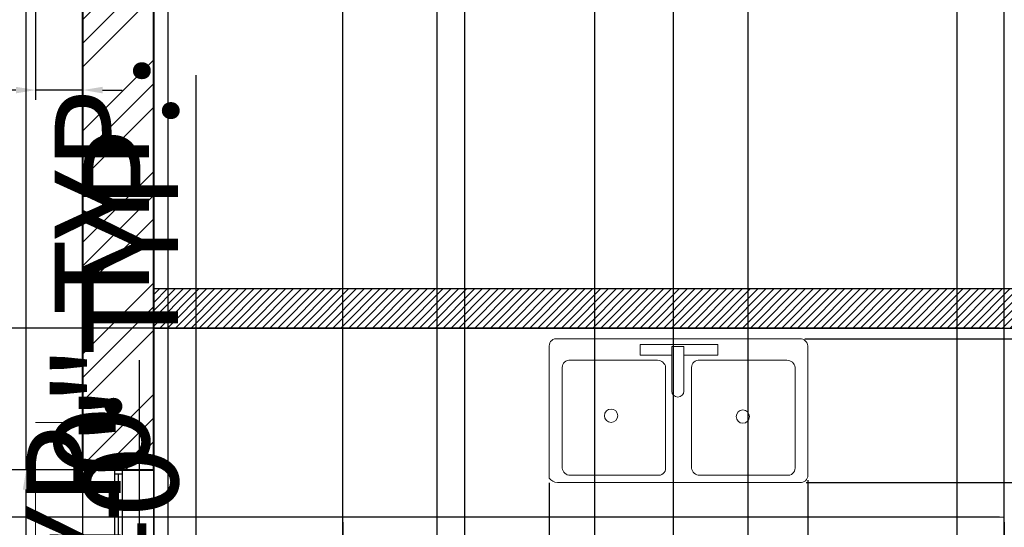
# Model space of a CAD drawing. Units: inches. Extents: x 2386 to 3029, y 792 to 1465.
# Tile 8 of 12: x 2463 to 2588, y 1205 to 1269. Entities that reach past the tile are written whole.
import ezdxf

# ---------------------------------------------------------------- set-up
doc = ezdxf.new("R2010")
doc.units = ezdxf.units.IN
doc.linetypes.add('ACAD_ISO02W100', pattern=[15, 12, -3])
for name, color, linetype, lineweight in [('A-DIMS', 1, 'Continuous', 18), ('A-FLOR-CASE', 6, 'Continuous', 18), ('A-FLOR-FIXT', 9, 'Continuous', 18), ('A-WALL-EXT', 7, 'Continuous', 40), ('A-WALL-INT', 9, 'Continuous', 30), ('A-WALL-PATT', 9, 'Continuous', 13), ('A-WINDOW', 4, 'Continuous', 25), ('A-WINDOW-OVHD', 4, 'ACAD_ISO02W100', 18)]:
    doc.layers.add(name, color=color, linetype=linetype, lineweight=lineweight)
doc.styles.get("Standard").update_dxf_attribs({"font": 'arial.ttf'})
doc.dimstyles.new('ISO-25', dxfattribs={"dimtxt": 12, "dimasz": 2.5, "dimexe": 1.25, "dimexo": 0.625, "dimtad": 1, "dimlunit": 4, "dimtxsty": 'Standard', "dimcen": 2.5, "dimadec": 0, "dimazin": 0, "dimtfac": 1, "dimtmove": 0, "dimatfit": 3, "dimfxl": 1, "dimarcsym": 0})

# ---------------------------------------------------------------- blocks, each defined once
blk = doc.blocks.new('WINDOW-48IN')
for p, q in [((0, 9), (48, 9)), ((0, 0), (0, 9)), ((48, 9), (48, 0)), ((48, 5), (0, 5)), ((48, 4), (0, 4)), ((0.5, 4), (0.5, 5)), ((47.5, 4.5), (0.5, 4.5)), ((47.5, 5), (47.5, 4)), ((48, 0), (0, 0))]:
    blk.add_line(p, q)
blk = doc.blocks.new('WINDOW-HOOD-48IN')
for p, q in [((0, 0), (0, 6)), ((60, 6), (60, 0)), ((60, 0), (0, 0))]:
    blk.add_line(p, q)
blk = doc.blocks.new('*D38')
at = {"layer": 'A-DIMS', "color": 0, "lineweight": -2, "transparency": 16777216}
for p, q in [((2471.82, 1342.95), (2483.24, 1342.95)), ((2481.99, 1340.45), (2481.99, 1273.45)), ((2471.82, 1270.95), (2483.24, 1270.95)), ((2481.99, 1270.95), (2481.99, 1095.04))]:
    blk.add_line(p, q, dxfattribs=at)
at = {"layer": 'A-DIMS', "color": 0, "transparency": 16777216}
for points in [[(2481.57, 1340.45), (2482.41, 1340.45), (2481.99, 1342.95)], [(2481.57, 1273.45), (2482.41, 1273.45), (2481.99, 1270.95)]]:
    blk.add_solid(points, dxfattribs=at)
at = {"layer": 'Defpoints', "color": 0, "transparency": 16777216}
for p in [(2471.19, 1342.95), (2471.19, 1270.95), (2481.99, 1270.95)]:
    blk.add_point(p, dxfattribs=at)
at = {"layer": 'A-DIMS', "color": 0, "transparency": 16777216, "insert": (2475.16, 1181.74), "char_height": 12, "attachment_point": 5, "rotation": 90}
blk.add_mtext('HOOD W-01 6\'-0" TYP.', dxfattribs=at)
blk = doc.blocks.new('*D39')
at = {"layer": 'A-DIMS', "color": 0, "lineweight": -2, "transparency": 16777216}
for p, q in [((2465.19, 1270.32), (2465.19, 1258.9)), ((2471.19, 1270.32), (2471.19, 1258.9)), ((2462.69, 1260.15), (2385.79, 1260.15)), ((2471.19, 1260.15), (2465.19, 1260.15)), ((2473.69, 1260.15), (2476.19, 1260.15))]:
    blk.add_line(p, q, dxfattribs=at)
at = {"layer": 'A-DIMS', "color": 0, "transparency": 16777216}
for points in [[(2462.69, 1260.56), (2462.69, 1259.73), (2465.19, 1260.15)], [(2473.69, 1260.56), (2473.69, 1259.73), (2471.19, 1260.15)]]:
    blk.add_solid(points, dxfattribs=at)
at = {"layer": 'Defpoints', "color": 0, "transparency": 16777216}
for p in [(2465.19, 1270.95), (2471.19, 1270.95), (2465.19, 1260.15)]:
    blk.add_point(p, dxfattribs=at)
at = {"layer": 'A-DIMS', "color": 0, "transparency": 16777216, "insert": (2422.99, 1266.9), "char_height": 12, "attachment_point": 5}
blk.add_mtext('0\'-6" TYP.', dxfattribs=at)
blk = doc.blocks.new('*D40')
at = {"layer": 'A-DIMS', "color": 0, "lineweight": -2, "transparency": 16777216}
for p, q in [((2463.99, 1211.95), (2463.99, 1334.04)), ((2470.57, 1211.95), (2462.74, 1211.95)), ((2463.99, 1166.45), (2463.99, 1209.45)), ((2470.57, 1163.95), (2462.74, 1163.95))]:
    blk.add_line(p, q, dxfattribs=at)
at = {"layer": 'A-DIMS', "color": 0, "transparency": 16777216}
for points in [[(2463.57, 1209.45), (2464.41, 1209.45), (2463.99, 1211.95)], [(2463.57, 1166.45), (2464.41, 1166.45), (2463.99, 1163.95)]]:
    blk.add_solid(points, dxfattribs=at)
at = {"layer": 'Defpoints', "color": 0, "transparency": 16777216}
for p in [(2463.99, 1211.95), (2471.19, 1211.95), (2471.19, 1163.95)]:
    blk.add_point(p, dxfattribs=at)
at = {"layer": 'A-DIMS', "color": 0, "transparency": 16777216, "insert": (2457.24, 1274.25), "char_height": 12, "attachment_point": 5, "rotation": 90}
blk.add_mtext('W-02 4\'-0" TYP.', dxfattribs=at)
blk = doc.blocks.new('*D44')
at = {"layer": 'A-DIMS', "color": 0, "lineweight": -2, "transparency": 16777216}
for p, q in [((2485.59, 1139.95), (2485.59, 1262.04)), ((2480.82, 1139.95), (2486.84, 1139.95)), ((2485.59, 1106.45), (2485.59, 1137.45)), ((2480.82, 1103.95), (2486.84, 1103.95))]:
    blk.add_line(p, q, dxfattribs=at)
at = {"layer": 'A-DIMS', "color": 0, "transparency": 16777216}
for points in [[(2485.17, 1137.45), (2486.01, 1137.45), (2485.59, 1139.95)], [(2485.17, 1106.45), (2486.01, 1106.45), (2485.59, 1103.95)]]:
    blk.add_solid(points, dxfattribs=at)
at = {"layer": 'Defpoints', "color": 0, "transparency": 16777216}
for p in [(2480.19, 1139.95), (2485.59, 1139.95), (2480.19, 1103.95)]:
    blk.add_point(p, dxfattribs=at)
at = {"layer": 'A-DIMS', "color": 0, "transparency": 16777216, "insert": (2478.83, 1202.25), "char_height": 12, "attachment_point": 5, "rotation": 90}
blk.add_mtext('W-03 3\'-0" TYP.', dxfattribs=at)
blk = doc.blocks.new('*D46')
at = {"layer": 'A-DIMS', "color": 0, "lineweight": -2, "transparency": 16777216}
for p, q in [((2478.39, 1049.95), (2478.39, 1225.86)), ((2471.82, 1049.95), (2479.64, 1049.95)), ((2478.39, 1004.45), (2478.39, 1047.45)), ((2471.82, 1001.95), (2479.64, 1001.95))]:
    blk.add_line(p, q, dxfattribs=at)
at = {"layer": 'A-DIMS', "color": 0, "transparency": 16777216}
for points in [[(2477.97, 1047.45), (2478.81, 1047.45), (2478.39, 1049.95)], [(2477.97, 1004.45), (2478.81, 1004.45), (2478.39, 1001.95)]]:
    blk.add_solid(points, dxfattribs=at)
at = {"layer": 'Defpoints', "color": 0, "transparency": 16777216}
for p in [(2471.19, 1049.95), (2478.39, 1049.95), (2471.19, 1001.95)]:
    blk.add_point(p, dxfattribs=at)
at = {"layer": 'A-DIMS', "color": 0, "transparency": 16777216, "insert": (2471.55, 1139.15), "char_height": 12, "attachment_point": 5, "rotation": 90}
blk.add_mtext('HOOD W-03 4\'-0" TYP.', dxfattribs=at)
blk = doc.blocks.new('*D52')
at = {"layer": 'A-DIMS', "color": 0, "lineweight": -2, "transparency": 16777216}
for p, q in [((2595.33, 1229.95), (2589.83, 1229.95)), ((2591.08, 1227.45), (2591.08, 1199.96)), ((2595.33, 1197.46), (2589.83, 1197.46)), ((2591.08, 1197.46), (2591.08, 1050.38))]:
    blk.add_line(p, q, dxfattribs=at)
at = {"layer": 'A-DIMS', "color": 0, "transparency": 16777216}
for points in [[(2590.67, 1227.45), (2591.5, 1227.45), (2591.08, 1229.95)], [(2590.67, 1199.96), (2591.5, 1199.96), (2591.08, 1197.46)]]:
    blk.add_solid(points, dxfattribs=at)
at = {"layer": 'Defpoints', "color": 0, "transparency": 16777216}
for p in [(2595.96, 1229.95), (2591.08, 1197.46), (2595.96, 1197.46)]:
    blk.add_point(p, dxfattribs=at)
at = {"layer": 'A-DIMS', "color": 0, "transparency": 16777216, "insert": (2584.25, 1122.67), "char_height": 12, "attachment_point": 5, "rotation": 90}
blk.add_mtext('REF. 2\'-8 1/2" TYP.', dxfattribs=at)
blk = doc.blocks.new('*D57')
at = {"layer": 'A-DIMS', "color": 0, "lineweight": -2, "transparency": 16777216}
for p, q in [((2546.19, 1008.57), (2546.19, 1427.9)), ((2582.19, 1008.57), (2582.19, 1427.9)), ((2548.69, 1426.65), (2579.69, 1426.65))]:
    blk.add_line(p, q, dxfattribs=at)
at = {"layer": 'A-DIMS', "color": 0, "transparency": 16777216}
for points in [[(2548.69, 1427.06), (2548.69, 1426.23), (2546.19, 1426.65)], [(2579.69, 1427.06), (2579.69, 1426.23), (2582.19, 1426.65)]]:
    blk.add_solid(points, dxfattribs=at)
at = {"layer": 'Defpoints', "color": 0, "transparency": 16777216}
for p in [(2582.19, 1426.65), (2546.19, 1007.95), (2582.19, 1007.95)]:
    blk.add_point(p, dxfattribs=at)
at = {"layer": 'A-DIMS', "color": 0, "transparency": 16777216, "insert": (2564.19, 1433.4), "char_height": 12, "attachment_point": 5}
blk.add_mtext('3\'-0"', dxfattribs=at)
blk = doc.blocks.new('*D65')
at = {"layer": 'A-DIMS', "color": 0, "lineweight": -2, "transparency": 16777216}
for p, q in [((2470.57, 1276.95), (2431.24, 1276.95)), ((2432.49, 1214.45), (2432.49, 1274.45)), ((2470.57, 1211.95), (2431.24, 1211.95))]:
    blk.add_line(p, q, dxfattribs=at)
at = {"layer": 'A-DIMS', "color": 0, "transparency": 16777216}
for points in [[(2432.07, 1274.45), (2432.91, 1274.45), (2432.49, 1276.95)], [(2432.07, 1214.45), (2432.91, 1214.45), (2432.49, 1211.95)]]:
    blk.add_solid(points, dxfattribs=at)
at = {"layer": 'Defpoints', "color": 0, "transparency": 16777216}
for p in [(2432.49, 1276.95), (2471.19, 1276.95), (2471.19, 1211.95)]:
    blk.add_point(p, dxfattribs=at)
at = {"layer": 'A-DIMS', "color": 0, "transparency": 16777216, "insert": (2425.76, 1244.45), "char_height": 12, "attachment_point": 5, "rotation": 90}
blk.add_mtext('5\'-5"', dxfattribs=at)
blk = doc.blocks.new('*D73')
at = {"layer": 'A-DIMS', "color": 0, "lineweight": -2, "transparency": 16777216}
for p, q in [((2519.68, 889.97), (2519.68, 1427.9)), ((2555.68, 889.97), (2555.68, 1427.9)), ((2522.18, 1426.65), (2553.18, 1426.65))]:
    blk.add_line(p, q, dxfattribs=at)
at = {"layer": 'A-DIMS', "color": 0, "transparency": 16777216}
for points in [[(2522.18, 1427.06), (2522.18, 1426.23), (2519.68, 1426.65)], [(2553.18, 1427.06), (2553.18, 1426.23), (2555.68, 1426.65)]]:
    blk.add_solid(points, dxfattribs=at)
at = {"layer": 'Defpoints', "color": 0, "transparency": 16777216}
for p in [(2555.68, 1426.65), (2519.68, 889.35), (2555.68, 889.35)]:
    blk.add_point(p, dxfattribs=at)
at = {"layer": 'A-DIMS', "color": 0, "transparency": 16777216, "insert": (2537.68, 1433.4), "char_height": 12, "attachment_point": 5}
blk.add_mtext('3\'-0"', dxfattribs=at)
blk = doc.blocks.new('*D75')
at = {"layer": 'A-DIMS', "color": 0, "lineweight": -2, "transparency": 16777216}
for p, q in [((2929.89, 1195.39), (2929.89, 1229.91)), ((2498.82, 1195.39), (2931.14, 1195.39)), ((2929.89, 1177.89), (2929.89, 1192.89)), ((2498.82, 1175.39), (2931.14, 1175.39))]:
    blk.add_line(p, q, dxfattribs=at)
at = {"layer": 'A-DIMS', "color": 0, "transparency": 16777216}
for points in [[(2929.47, 1192.89), (2930.31, 1192.89), (2929.89, 1195.39)], [(2929.47, 1177.89), (2930.31, 1177.89), (2929.89, 1175.39)]]:
    blk.add_solid(points, dxfattribs=at)
at = {"layer": 'Defpoints', "color": 0, "transparency": 16777216}
for p in [(2498.19, 1195.39), (2929.89, 1195.39), (2498.19, 1175.39)]:
    blk.add_point(p, dxfattribs=at)
at = {"layer": 'A-DIMS', "color": 0, "transparency": 16777216, "insert": (2923.14, 1213.9), "char_height": 12, "attachment_point": 5, "rotation": 90}
blk.add_mtext('1\'-8"', dxfattribs=at)
blk = doc.blocks.new('*D78')
at = {"layer": 'A-DIMS', "color": 0, "lineweight": -2, "transparency": 16777216}
for p, q in [((2516.19, 1054.57), (2516.19, 1427.9)), ((2536.19, 1044.57), (2536.19, 1427.9)), ((2518.69, 1426.65), (2533.69, 1426.65)), ((2536.19, 1426.65), (2570.71, 1426.65))]:
    blk.add_line(p, q, dxfattribs=at)
at = {"layer": 'A-DIMS', "color": 0, "transparency": 16777216}
for points in [[(2518.69, 1427.06), (2518.69, 1426.23), (2516.19, 1426.65)], [(2533.69, 1427.06), (2533.69, 1426.23), (2536.19, 1426.65)]]:
    blk.add_solid(points, dxfattribs=at)
at = {"layer": 'Defpoints', "color": 0, "transparency": 16777216}
for p in [(2536.19, 1426.65), (2516.19, 1053.95), (2536.19, 1043.95)]:
    blk.add_point(p, dxfattribs=at)
at = {"layer": 'A-DIMS', "color": 0, "transparency": 16777216, "insert": (2554.7, 1433.4), "char_height": 12, "attachment_point": 5}
blk.add_mtext('1\'-8"', dxfattribs=at)
blk = doc.blocks.new('*D93')
at = {"layer": 'A-DIMS', "color": 0, "lineweight": -2, "transparency": 16777216}
for p, q in [((2432.49, 1229.95), (2432.49, 1265.8)), ((2587.57, 1229.95), (2431.24, 1229.95)), ((2432.49, 1208.45), (2432.49, 1227.45)), ((2587.57, 1205.95), (2431.24, 1205.95))]:
    blk.add_line(p, q, dxfattribs=at)
at = {"layer": 'A-DIMS', "color": 0, "transparency": 16777216}
for points in [[(2432.07, 1227.45), (2432.91, 1227.45), (2432.49, 1229.95)], [(2432.07, 1208.45), (2432.91, 1208.45), (2432.49, 1205.95)]]:
    blk.add_solid(points, dxfattribs=at)
at = {"layer": 'Defpoints', "color": 0, "transparency": 16777216}
for p in [(2432.49, 1229.95), (2588.19, 1229.95), (2588.19, 1205.95)]:
    blk.add_point(p, dxfattribs=at)
at = {"layer": 'A-DIMS', "color": 0, "transparency": 16777216, "insert": (2425.74, 1249.12), "char_height": 12, "attachment_point": 5, "rotation": 90}
blk.add_mtext('2\'-0"', dxfattribs=at)
blk = doc.blocks.new('*D94')
at = {"layer": 'A-DIMS', "color": 0, "lineweight": -2, "transparency": 16777216}
for p, q in [((2504.19, 1205.32), (2504.19, 808)), ((2588.19, 1205.32), (2588.19, 808)), ((2506.69, 809.25), (2585.69, 809.25))]:
    blk.add_line(p, q, dxfattribs=at)
at = {"layer": 'A-DIMS', "color": 0, "transparency": 16777216}
for points in [[(2506.69, 809.66), (2506.69, 808.83), (2504.19, 809.25)], [(2585.69, 809.66), (2585.69, 808.83), (2588.19, 809.25)]]:
    blk.add_solid(points, dxfattribs=at)
at = {"layer": 'Defpoints', "color": 0, "transparency": 16777216}
for p in [(2504.19, 1205.95), (2588.19, 1205.95), (2588.19, 809.25)]:
    blk.add_point(p, dxfattribs=at)
at = {"layer": 'A-DIMS', "color": 0, "transparency": 16777216, "insert": (2546.19, 816), "char_height": 12, "attachment_point": 5}
blk.add_mtext('7\'-0"', dxfattribs=at)
blk = doc.blocks.new('*D95')
at = {"layer": 'A-DIMS', "color": 0, "lineweight": -2, "transparency": 16777216}
for p, q in [((2480.19, 1146.57), (2480.19, 1427.9)), ((2504.19, 1146.57), (2504.19, 1427.9)), ((2482.69, 1426.65), (2501.69, 1426.65)), ((2504.19, 1426.65), (2540.04, 1426.65))]:
    blk.add_line(p, q, dxfattribs=at)
at = {"layer": 'A-DIMS', "color": 0, "transparency": 16777216}
for points in [[(2482.69, 1427.06), (2482.69, 1426.23), (2480.19, 1426.65)], [(2501.69, 1427.06), (2501.69, 1426.23), (2504.19, 1426.65)]]:
    blk.add_solid(points, dxfattribs=at)
at = {"layer": 'Defpoints', "color": 0, "transparency": 16777216}
for p in [(2504.19, 1426.65), (2480.19, 1145.95), (2504.19, 1145.95)]:
    blk.add_point(p, dxfattribs=at)
at = {"layer": 'A-DIMS', "color": 0, "transparency": 16777216, "insert": (2523.37, 1433.4), "char_height": 12, "attachment_point": 5}
blk.add_mtext('2\'-0"', dxfattribs=at)
blk = doc.blocks.new('*D96')
at = {"layer": 'A-DIMS', "color": 0, "lineweight": -2, "transparency": 16777216}
for p, q in [((2516.19, 893.57), (2516.19, 1427.9)), ((2588.19, 893.57), (2588.19, 1427.9)), ((2518.69, 1426.65), (2585.69, 1426.65))]:
    blk.add_line(p, q, dxfattribs=at)
at = {"layer": 'A-DIMS', "color": 0, "transparency": 16777216}
for points in [[(2518.69, 1427.06), (2518.69, 1426.23), (2516.19, 1426.65)], [(2585.69, 1427.06), (2585.69, 1426.23), (2588.19, 1426.65)]]:
    blk.add_solid(points, dxfattribs=at)
at = {"layer": 'Defpoints', "color": 0, "transparency": 16777216}
for p in [(2588.19, 1426.65), (2516.19, 892.95), (2588.19, 892.95)]:
    blk.add_point(p, dxfattribs=at)
at = {"layer": 'A-DIMS', "color": 0, "transparency": 16777216, "insert": (2552.19, 1433.4), "char_height": 12, "attachment_point": 5}
blk.add_mtext('6\'-0"', dxfattribs=at)
blk = doc.blocks.new('*D99')
at = {"layer": 'A-DIMS', "color": 0, "lineweight": -2, "transparency": 16777216}
for p, q in [((2530.41, 1210.29), (2530.41, 808)), ((2563.26, 1210.63), (2563.26, 808)), ((2532.91, 809.25), (2560.76, 809.25)), ((2563.26, 809.25), (2599.11, 809.25))]:
    blk.add_line(p, q, dxfattribs=at)
at = {"layer": 'A-DIMS', "color": 0, "transparency": 16777216}
for points in [[(2532.91, 809.66), (2532.91, 808.83), (2530.41, 809.25)], [(2560.76, 809.66), (2560.76, 808.83), (2563.26, 809.25)]]:
    blk.add_solid(points, dxfattribs=at)
at = {"layer": 'Defpoints', "color": 0, "transparency": 16777216}
for p in [(2530.41, 1210.91), (2563.26, 1211.26), (2563.26, 809.25)]:
    blk.add_point(p, dxfattribs=at)
at = {"layer": 'A-DIMS', "color": 0, "transparency": 16777216, "insert": (2582.43, 816), "char_height": 12, "attachment_point": 5}
blk.add_mtext('2\'-9"', dxfattribs=at)
blk = doc.blocks.new('*D100')
at = {"layer": 'A-DIMS', "color": 0, "lineweight": -2, "transparency": 16777216}
for p, q in [((2562.86, 1228.59), (2931.14, 1228.59)), ((2929.89, 1226.09), (2929.89, 1212.84)), ((2563.05, 1210.34), (2931.14, 1210.34)), ((2929.89, 1210.34), (2929.89, 1147.86))]:
    blk.add_line(p, q, dxfattribs=at)
at = {"layer": 'A-DIMS', "color": 0, "transparency": 16777216}
for points in [[(2929.47, 1226.09), (2930.31, 1226.09), (2929.89, 1228.59)], [(2929.47, 1212.84), (2930.31, 1212.84), (2929.89, 1210.34)]]:
    blk.add_solid(points, dxfattribs=at)
at = {"layer": 'Defpoints', "color": 0, "transparency": 16777216}
for p in [(2562.24, 1228.59), (2562.43, 1210.34), (2929.89, 1210.34)]:
    blk.add_point(p, dxfattribs=at)
at = {"layer": 'A-DIMS', "color": 0, "transparency": 16777216, "insert": (2923.06, 1177.85), "char_height": 12, "attachment_point": 5, "rotation": 90}
blk.add_mtext('1\'-6 1/2"', dxfattribs=at)
blk = doc.blocks.new('*D101')
at = {"layer": 'A-DIMS', "color": 0, "lineweight": -2, "transparency": 16777216}
for p, q in [((2929.89, 1175.39), (2929.89, 1239.21)), ((2480.82, 1175.39), (2931.14, 1175.39)), ((2929.89, 1148.45), (2929.89, 1172.89)), ((2480.82, 1145.95), (2931.14, 1145.95))]:
    blk.add_line(p, q, dxfattribs=at)
at = {"layer": 'A-DIMS', "color": 0, "transparency": 16777216}
for points in [[(2929.47, 1172.89), (2930.31, 1172.89), (2929.89, 1175.39)], [(2929.47, 1148.45), (2930.31, 1148.45), (2929.89, 1145.95)]]:
    blk.add_solid(points, dxfattribs=at)
at = {"layer": 'Defpoints', "color": 0, "transparency": 16777216}
for p in [(2480.19, 1175.39), (2929.89, 1175.39), (2480.19, 1145.95)]:
    blk.add_point(p, dxfattribs=at)
at = {"layer": 'A-DIMS', "color": 0, "transparency": 16777216, "insert": (2923.06, 1208.55), "char_height": 12, "attachment_point": 5, "rotation": 90}
blk.add_mtext('2\'-5 1/2"', dxfattribs=at)

msp = doc.modelspace()

# ---------------------------------------------------------------- hatches: boundary and pattern name
at = {"layer": 'A-WALL-PATT'}
h = msp.add_hatch(dxfattribs=at)
h.set_pattern_fill('GOST_GROUND', color=256)
h.paths.add_polyline_path([(2480.19, 1276.948), (2471.19, 1276.948), (2471.19, 1211.948), (2480.19, 1211.948)])
h.paths.add_polyline_path([(2480.19, 1378.948), (2510.19, 1378.948), (2510.19, 1378.969), (2523.779, 1378.969), (2580.602, 1378.959), (2580.602, 1378.969), (2594.19, 1378.969), (2642.19, 1378.948), (2642.19, 1387.948), (2471.19, 1387.948), (2471.19, 1336.948), (2480.19, 1336.948)])
h.paths.add_polyline_path([(2891.19, 1387.948), (2666.19, 1387.948), (2666.19, 1378.948), (2882.19, 1378.948), (2882.19, 1355.948), (2891.19, 1355.948)])
h.paths.add_polyline_path([(2891.19, 1331.948), (2882.19, 1331.948), (2882.19, 1331.449), (2882.19, 1261.948), (2891.19, 1261.948)])
h.paths.add_polyline_path([(2891.19, 1201.948), (2882.19, 1201.948), (2882.19, 1189.948), (2882.19, 1159.948), (2882.19, 1117.948), (2891.19, 1117.948)])
h.paths.add_polyline_path([(2891.19, 1057.948), (2882.19, 1057.948), (2882.19, 856.948), (2882.19, 847.948), (2891.19, 847.948)])
h.paths.add_polyline_path([(2594.19, 856.948), (2558.19, 856.948), (2558.19, 847.948), (2594.19, 847.948)])
h.paths.add_polyline_path([(2510.19, 856.948), (2480.19, 856.948), (2480.19, 905.448), (2471.19, 905.448), (2471.19, 847.948), (2510.19, 847.948)])
h.paths.add_polyline_path([(2480.19, 1007.948), (2471.19, 1007.948), (2471.19, 953.448), (2480.19, 953.448)])
h.paths.add_polyline_path([(2480.19, 1103.948), (2471.19, 1103.948), (2471.19, 1043.948), (2480.19, 1043.948)])
h = msp.add_hatch(dxfattribs=at)
h.set_pattern_fill('JIS_WOOD', color=256)
h.paths.add_polyline_path([(2624.19, 1229.948), (2624.19, 1145.948), (2618.19, 1145.948), (2618.19, 1140.548), (2618.19, 1139.948), (2630.19, 1139.948), (2630.19, 1240.948), (2624.19, 1240.948), (2624.19, 1234.948), (2480.19, 1234.948), (2480.19, 1229.948)])
h.paths.add_polyline_path([(2582.19, 1139.948), (2582.19, 1145.948), (2480.19, 1145.948), (2480.19, 1139.948)], flags=17)
h.paths.add_polyline_path([(2480.19, 1007.948), (2480.19, 1001.948), (2546.19, 1001.948), (2546.19, 1007.348), (2546.19, 1007.948)])
h.paths.add_polyline_path([(2594.19, 1007.948), (2582.19, 1007.948), (2582.19, 1001.948), (2588.19, 1001.948), (2588.19, 856.948), (2594.19, 856.948), (2594.19, 914.948), (2606.19, 914.948), (2606.19, 920.948), (2594.19, 920.948)])
h.paths.add_polyline_path([(2738.19, 1015.948), (2882.19, 1015.948), (2882.19, 1021.948), (2738.19, 1021.948), (2738.19, 1111.948), (2732.19, 1111.948), (2732.19, 920.948), (2720.19, 920.948), (2720.19, 914.948), (2732.19, 914.948), (2732.19, 856.948), (2738.19, 856.948)])
h.paths.add_polyline_path([(2660.19, 914.948), (2660.19, 920.948), (2648.19, 920.948), (2648.19, 914.948)])
h.paths.add_polyline_path([(2738.19, 1159.948), (2738.19, 1165.948), (2737.59, 1165.948), (2732.19, 1165.948), (2732.19, 1147.948), (2737.59, 1147.948), (2738.19, 1147.948), (2738.19, 1153.948), (2882.19, 1153.948), (2882.19, 1159.948)])
h.paths.add_polyline_path([(2732.19, 1201.948), (2738.19, 1201.948), (2738.19, 1303.948), (2774.19, 1303.948), (2774.19, 1308.948), (2768.19, 1308.948), (2768.19, 1378.948), (2762.19, 1378.948), (2762.19, 1308.948), (2726.19, 1308.948), (2726.19, 1303.948), (2732.19, 1303.948)])
h.paths.add_polyline_path([(2696.19, 1303.948), (2696.19, 1308.948), (2630.19, 1308.948), (2630.19, 1378.948), (2624.19, 1378.948), (2624.19, 1276.948), (2630.19, 1276.948), (2630.19, 1303.948)])

# ---------------------------------------------------------------- linework, layer by layer
at = {"layer": 'A-FLOR-CASE'}
msp.add_lwpolyline([(2504.19, 1145.948), (2504.19, 1205.948), (2588.19, 1205.948), (2588.19, 1229.948)], dxfattribs=at)
at = {"layer": 'A-FLOR-FIXT'}
for p, q in [((2531.439, 1228.595), (2562.236, 1228.595)), ((2551.808, 1227.852), (2541.953, 1227.852)), ((2541.953, 1227.852), (2541.953, 1226.485)), ((2551.808, 1226.485), (2551.808, 1227.852)), ((2530.413, 1210.915), (2530.407, 1227.682)), ((2545.975, 1227.616), (2545.975, 1221.956)), ((2547.504, 1227.616), (2545.975, 1227.616)), ((2547.504, 1221.956), (2547.504, 1227.616)), ((2563.257, 1227.682), (2563.257, 1211.257)), ((2533.076, 1225.857), (2544.163, 1225.857)), ((2541.953, 1226.485), (2545.975, 1226.485)), ((2547.504, 1226.485), (2551.808, 1226.485)), ((2549.501, 1225.857), (2560.588, 1225.857)), ((2532.05, 1212.17), (2532.05, 1224.945)), ((2545.19, 1224.945), (2545.19, 1212.17)), ((2548.475, 1212.17), (2548.475, 1224.945)), ((2561.615, 1224.945), (2561.615, 1212.17)), ((2562.231, 1210.345), (2531.439, 1210.345)), ((2544.163, 1211.257), (2533.076, 1211.257)), ((2560.588, 1211.257), (2549.501, 1211.257))]:
    msp.add_line(p, q, dxfattribs=at)
for centre in [(2538.254, 1218.824), (2554.988, 1218.709)]:
    msp.add_circle(centre, 0.844, dxfattribs=at)
for centre, radius, start, end in [((2531.326, 1227.682), 0.919, 82.92547, 180.01993), ((2562.236, 1227.567), 1.027, 6.40919, 90.00001), ((2532.968, 1224.945), 0.919, 83.26708, 179.99999), ((2544.163, 1224.823), 1.034, 6.73295, 89.99997), ((2549.393, 1224.945), 0.919, 83.26708, 179.99999), ((2560.588, 1224.823), 1.034, 6.73295, 89.99997), ((2546.74, 1221.956), 0.765, 180, 0), ((2533.076, 1212.291), 1.034, 186.73295, 269.99997), ((2544.271, 1212.17), 0.919, 263.26708, 359.99999), ((2549.501, 1212.291), 1.034, 186.73295, 269.99997), ((2560.696, 1212.17), 0.919, 263.26708, 359.99999), ((2531.439, 1211.554), 1.209, 211.89079, 270), ((2562.338, 1211.257), 0.919, 263.26708, 359.99999)]:
    msp.add_arc(centre, radius, start, end, dxfattribs=at)
at = {"layer": 'A-WALL-EXT'}
for p, q in [((2471.19, 1211.948), (2471.19, 1276.948)), ((2480.19, 1211.948), (2480.19, 1276.948)), ((2471.19, 1211.948), (2480.19, 1211.948)), ((2471.19, 1211.948), (2480.19, 1211.948))]:
    msp.add_line(p, q, dxfattribs=at)
at = {"layer": 'A-WALL-INT'}
for p, q in [((2480.19, 1234.948), (2624.19, 1234.948)), ((2480.19, 1229.948), (2624.19, 1229.948))]:
    msp.add_line(p, q, dxfattribs=at)

# ---------------------------------------------------------------- block references
at = {"layer": 'A-WINDOW', "rotation": 89.9999999997146}
msp.add_blockref('WINDOW-48IN', (2480.19, 1163.948), dxfattribs=at)
at = {"layer": 'A-WINDOW-OVHD', "rotation": 269.9999999991061}
msp.add_blockref('WINDOW-HOOD-48IN', (2465.19, 1217.948), dxfattribs=at)

# ---------------------------------------------------------------- dimensions: what is measured, and where the dimension line sits
at = {"layer": 'A-DIMS'}
for base, p1, p2, picture, middle in [((2504.19, 1426.648), (2480.19, 1145.948), (2504.19, 1145.948), '*D95', (2523.367, 1433.4)), ((2536.19, 1426.648), (2516.19, 1053.948), (2536.19, 1043.948), '*D78', (2554.7, 1433.4)), ((2588.19, 1426.648), (2516.19, 892.948), (2588.19, 892.948), '*D96', (2552.19, 1433.4)), ((2555.676, 1426.648), (2519.676, 889.348), (2555.676, 889.348), '*D73', (2537.676, 1433.404)), ((2582.19, 1426.648), (2546.19, 1007.948), (2582.19, 1007.948), '*D57', (2564.19, 1433.404)), ((2563.257, 809.248), (2530.413, 1210.915), (2563.257, 1211.257), '*D99', (2582.434, 816)), ((2588.19, 809.248), (2504.19, 1205.948), (2588.19, 1205.948), '*D94', (2546.19, 816))]:
    dim = msp.add_linear_dim(base=base, p1=p1, p2=p2, dimstyle='ISO-25', override={"dimdec": 1, "dimlfac": 1, "dimrnd": 0, "dimzin": 1, "dimdsep": 46, "dimlunit": 4, "dimfrac": 2}, dxfattribs=at)
    dim.commit()
    dim.dimension.update_dxf_attribs({"geometry": picture, "text_midpoint": middle})
for base, p1, p2, angle, text, picture, middle in [((2481.99, 1270.948), (2471.19, 1342.948), (2471.19, 1270.948), 270, 'HOOD W-01 <> TYP.', '*D38', (2475.156, 1181.744)), ((2463.99, 1211.948), (2471.19, 1163.948), (2471.19, 1211.948), 90, 'W-02 <> TYP.', '*D40', (2457.238, 1274.246)), ((2465.19, 1260.148), (2471.19, 1270.948), (2465.19, 1270.948), 180, '<> TYP.', '*D39', (2422.992, 1266.9)), ((2485.59, 1139.948), (2480.19, 1103.948), (2480.19, 1139.948), 90, 'W-03 <> TYP.', '*D44', (2478.834, 1202.246)), ((2591.083, 1197.463), (2595.956, 1229.948), (2595.956, 1197.463), 270, 'REF. <> TYP.', '*D52', (2584.253, 1122.673)), ((2478.39, 1049.948), (2471.19, 1001.948), (2471.19, 1049.948), 90, 'HOOD W-03 <> TYP.', '*D46', (2471.552, 1139.152))]:
    dim = msp.add_linear_dim(base=base, p1=p1, p2=p2, angle=angle, text=text, dimstyle='ISO-25', override={"dimdec": 1, "dimlfac": 1, "dimrnd": 0, "dimzin": 1, "dimdsep": 46, "dimlunit": 4, "dimfrac": 2}, dxfattribs=at)
    dim.commit()
    dim.dimension.update_dxf_attribs({"geometry": picture, "text_midpoint": middle})
for base, p1, p2, picture, middle in [((2432.49, 1276.948), (2471.19, 1211.948), (2471.19, 1276.948), '*D65', (2425.763, 1244.448)), ((2432.49, 1229.948), (2588.19, 1205.948), (2588.19, 1229.948), '*D93', (2425.738, 1249.125)), ((2929.89, 1175.392), (2480.19, 1145.948), (2480.19, 1175.392), '*D101', (2923.06, 1208.55)), ((2929.89, 1195.392), (2498.19, 1175.392), (2498.19, 1195.392), '*D75', (2923.138, 1213.902)), ((2929.89, 1210.342), (2562.236, 1228.595), (2562.425, 1210.342), '*D100', (2923.06, 1177.852))]:
    dim = msp.add_linear_dim(base=base, p1=p1, p2=p2, angle=90, dimstyle='ISO-25', override={"dimdec": 1, "dimlfac": 1, "dimrnd": 0, "dimzin": 1, "dimdsep": 46, "dimlunit": 4, "dimfrac": 2}, dxfattribs=at)
    dim.commit()
    dim.dimension.update_dxf_attribs({"geometry": picture, "text_midpoint": middle})

doc.saveas('drawing.dxf')
